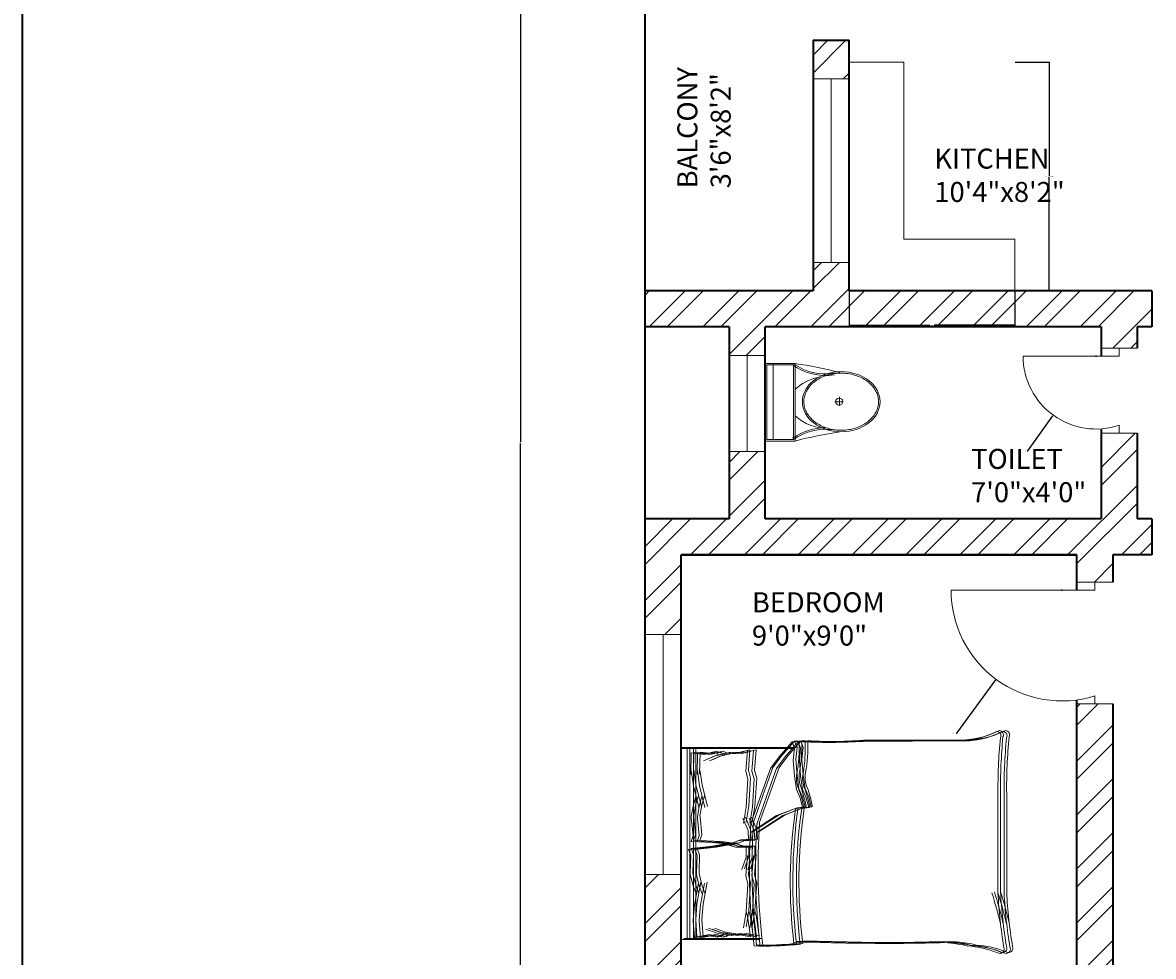
# Model space of a CAD drawing. Units: inches. Extents: x 1955 to 3324, y 980 to 3129.
# Tile 3 of 11: x 1955 to 2237, y 2048 to 2282. Entities that reach past the tile are written whole.
import ezdxf

# ---------------------------------------------------------------- set-up
doc = ezdxf.new("R2010")
doc.units = ezdxf.units.IN
for name, color, linetype, lineweight in [('A-ANNO-DIMS', 2, 'Continuous', 18), ('A-ANNO-TTLB', 7, 'Continuous', 35), ('A-AREA-IDEN', 7, 'Continuous', 18), ('A-DOOR', 3, 'Continuous', 18), ('A-FLOR-CASE', 8, 'Continuous', 18), ('A-FLOR-FIXT', 9, 'Continuous', 18), ('A-FURN', 8, 'Continuous', 18), ('A-GLAZ', 4, 'Continuous', 18), ('A-WALL', 7, 'Continuous', 35), ('A-WALL-PATT', 252, 'Continuous', 13)]:
    doc.layers.add(name, color=color, linetype=linetype, lineweight=lineweight)
doc.styles.get("Standard").update_dxf_attribs({"font": 'arial.ttf'})
doc.dimstyles.get("Standard").update_dxf_attribs({"dimtxt": 0.18, "dimasz": 0.18, "dimexe": 0.18, "dimexo": 0.0625, "dimgap": 0.09, "dimtad": 0, "dimtih": 1, "dimtoh": 1, "dimdec": 4, "dimzin": 0, "dimdsep": 46, "dimtxsty": 'Standard', "dimcen": 0.09, "dimadec": 0, "dimazin": 0, "dimtfac": 1, "dimtdec": 4, "dimtofl": 0, "dimtmove": 0, "dimatfit": 3, "dimfxl": 1, "dimtolj": 1, "dimtzin": 0, "dimarcsym": 0})

# ---------------------------------------------------------------- blocks, each defined once
blk = doc.blocks.new('A$C31115884')
for p, q in [((283.1, 497.7), (223.4, 497.7)), ((257.5, 466.4), (257.5, 523.2)), ((0, 200), (0, 0)), ((520, 200), (0, 200)), ((10, 190), (10, 10)), ((510, 190), (10, 190)), ((510, 10), (510, 190)), ((520, 0), (520, 200)), ((510, 54.5), (0, 54.5)), ((10, 10), (510, 10)), ((0, 0), (520, 0))]:
    blk.add_line(p, q)
blk.add_circle((255.6, 496.4), 23.6)
for centre, radius, start, end in [((2777.7, -204.6), 2807, 165.4549, 171.71327), ((-294.5, 403.3), 364.7, 324.20913, 9.34987), ((-294.5, 403.3), 374.7, 324.20913, 9.34987), ((805.8, 403.3), 364.7, 170.65013, 215.79087), ((3237, 905), 2807, 188.28673, 194.5451), ((139.5, 406.2), 293.5, 315.84364, 2.65635), ((805.8, 403.3), 374.7, 179.20365, 215.79087), ((383.6, 406.2), 293.5, 190.27735, 224.15636)]:
    blk.add_arc(centre, radius, start, end)
blk.add_ellipse((256.2, 509.9), major_axis=(0, -260.7), ratio=0.772727)
blk.add_open_spline([(256.2, 259.2), (263.1, 259.2), (270, 259.7), (287.8, 262.3), (298.7, 265.1), (319.9, 273.1), (330.2, 278.4), (350.1, 291.1), (359.7, 298.7), (377.7, 315.9), (386.2, 325.5), (401.7, 346.6), (408.8, 358.1), (421.3, 382.5), (426.8, 395.5), (435.9, 422.4), (439.5, 436.4), (444.8, 465.1), (446.5, 479.7), (447.9, 509.2), (447.6, 524), (445, 553.3), (442.7, 567.8), (436.3, 596), (432.1, 609.7), (421.9, 636), (416, 648.6), (402.5, 672.1), (395, 683), (378.6, 703), (369.8, 712.1), (351.1, 728), (341.3, 734.8), (320.9, 746.2), (310.4, 750.7), (288.9, 757.3), (278, 759.4), (256, 761), (245, 760.6), (223.1, 757.2), (212.3, 754.3), (191.1, 746.1), (180.8, 740.7), (160.9, 727.8), (151.4, 720.1), (133.5, 702.7), (125.1, 693), (109.6, 671.7), (102.6, 660.2), (90.2, 635.7), (84.9, 622.7), (76, 595.6), (72.4, 581.6), (67.2, 552.9), (65.6, 538.2), (64.4, 508.8), (64.8, 494), (67.5, 464.7), (69.9, 450.2), (76.6, 422), (80.8, 408.3), (91.1, 382.2), (97.2, 369.7), (110.8, 346.3), (118.4, 335.4), (134.8, 315.6), (143.7, 306.7), (162.4, 290.9), (172.3, 284.2), (192.8, 273), (203.3, 268.6), (224.8, 262.2), (235.8, 260.2), (249.9, 259.3), (253, 259.2), (256.2, 259.2)], degree=3, knots=[0, 0, 0, 0, 0.110105, 0.110105, 0.285049, 0.285049, 0.459994, 0.459994, 0.634938, 0.634938, 0.809882, 0.809882, 0.984827, 0.984827, 1.159771, 1.159771, 1.334715, 1.334715, 1.50966, 1.50966, 1.684604, 1.684604, 1.859549, 1.859549, 2.034493, 2.034493, 2.209437, 2.209437, 2.384382, 2.384382, 2.559326, 2.559326, 2.73427, 2.73427, 2.909215, 2.909215, 3.084159, 3.084159, 3.259103, 3.259103, 3.434048, 3.434048, 3.608992, 3.608992, 3.783936, 3.783936, 3.958881, 3.958881, 4.133825, 4.133825, 4.30877, 4.30877, 4.483714, 4.483714, 4.658658, 4.658658, 4.833603, 4.833603, 5.008547, 5.008547, 5.183491, 5.183491, 5.358436, 5.358436, 5.53338, 5.53338, 5.708324, 5.708324, 5.883269, 5.883269, 6.058213, 6.058213, 6.233158, 6.233158, 6.283185, 6.283185, 6.283185, 6.283185])
blk = doc.blocks.new('BED-WITH-PILLOWS')
for p, q in [((3.48, 63.33), (3.48, 81.44)), ((3.48, 63.33), (3.48, 81.44)), ((51.27, 81.44), (3.48, 81.44)), ((3.48, 79.91), (51.27, 79.91)), ((3.48, 79.91), (51.27, 79.91)), ((3.7, 62.69), (3.7, 80.8)), ((3.7, 62.69), (3.7, 80.8)), ((3.7, 79.27), (51.49, 79.27)), ((3.7, 79.27), (51.49, 79.27)), ((24.54, 78.99), (25.98, 79.57)), ((24.54, 78.99), (25.98, 79.57)), ((25.98, 79.57), (26.56, 74.22)), ((25.98, 79.57), (26.56, 74.22)), ((51.27, 81.44), (51.27, 54.83)), ((51.27, 81.44), (51.27, 54.83)), ((51.27, 81.44), (51.49, 81.44)), ((51.49, 81.44), (51.49, 80.8)), ((51.49, 80.8), (51.49, 54.19)), ((51.49, 80.8), (51.49, 54.19)), ((3.89, 78.13), (4.47, 74.95)), ((3.9, 78.11), (8.18, 78.43)), ((3.9, 78.11), (8.18, 78.43)), ((3.9, 78.13), (4.47, 74.95)), ((4.12, 77.49), (4.7, 74.31)), ((4.12, 77.49), (4.7, 74.31)), ((4.13, 77.47), (8.41, 77.8)), ((4.13, 77.47), (8.41, 77.8)), ((8.18, 78.43), (8.29, 78.42)), ((8.18, 78.43), (8.29, 78.42)), ((8.29, 78.42), (12.11, 78.13)), ((8.29, 78.42), (12.11, 78.13)), ((8.41, 77.8), (8.51, 77.78)), ((8.41, 77.8), (8.51, 77.78)), ((8.51, 77.78), (12.34, 77.49)), ((8.51, 77.78), (12.34, 77.49)), ((12.11, 78.13), (17.6, 77.12)), ((12.11, 78.13), (17.6, 77.12)), ((12.34, 77.49), (17.83, 76.48)), ((12.34, 77.49), (17.83, 76.48)), ((14.86, 77.69), (16.88, 78.42)), ((14.86, 77.69), (16.88, 78.42)), ((15.08, 77.05), (17.11, 77.78)), ((15.08, 77.05), (17.11, 77.78)), ((16.88, 78.42), (19.77, 79.14)), ((16.88, 78.42), (19.77, 79.14)), ((17.11, 77.78), (20, 78.5)), ((17.11, 77.78), (20, 78.5)), ((19.77, 79.14), (20.09, 79.14)), ((19.77, 79.14), (20.09, 79.14)), ((20, 78.5), (20.32, 78.5)), ((20, 78.5), (20.32, 78.5)), ((20.09, 79.14), (24.54, 78.99)), ((20.09, 79.14), (24.54, 78.99)), ((20.32, 78.5), (24.77, 78.36)), ((20.32, 78.5), (24.77, 78.36)), ((24.77, 78.36), (26.21, 78.93)), ((24.77, 78.36), (26.21, 78.93)), ((26.21, 78.93), (26.79, 73.58)), ((26.21, 78.93), (26.79, 73.58)), ((27.98, 78.95), (27.73, 73.58)), ((27.98, 78.95), (27.73, 73.58)), ((28.21, 78.31), (27.96, 72.94)), ((28.21, 78.31), (27.96, 72.94)), ((29.46, 78.46), (27.98, 78.95)), ((29.46, 78.46), (27.98, 78.95)), ((29.68, 77.83), (28.21, 78.31)), ((29.68, 77.83), (28.21, 78.31)), ((33.88, 78.89), (29.46, 78.46)), ((33.88, 78.89), (29.46, 78.46)), ((34.11, 78.25), (29.68, 77.83)), ((34.11, 78.25), (29.68, 77.83)), ((34.21, 78.91), (33.88, 78.89)), ((34.2, 78.91), (33.88, 78.89)), ((34.43, 78.27), (34.11, 78.25)), ((34.43, 78.27), (34.11, 78.25)), ((37.14, 78.36), (34.2, 78.91)), ((37.14, 78.36), (34.21, 78.91)), ((37.36, 77.73), (34.43, 78.27)), ((37.36, 77.73), (34.43, 78.27)), ((41.91, 78.37), (36.5, 77.02)), ((41.91, 78.37), (36.5, 77.02)), ((42.14, 77.73), (36.72, 76.38)), ((42.14, 77.73), (36.72, 76.38)), ((39.2, 77.77), (37.14, 78.36)), ((39.2, 77.77), (37.14, 78.36)), ((39.43, 77.13), (37.36, 77.73)), ((39.43, 77.13), (37.36, 77.73)), ((45.71, 78.9), (41.91, 78.37)), ((45.71, 78.9), (41.91, 78.37)), ((45.94, 78.26), (42.14, 77.73)), ((45.94, 78.26), (42.14, 77.73)), ((50.11, 78.89), (44.71, 78.98)), ((44.71, 78.98), (45.71, 78.9)), ((50.11, 78.89), (44.71, 78.98)), ((44.71, 78.98), (45.71, 78.9)), ((50.34, 78.25), (44.94, 78.34)), ((44.94, 78.34), (45.94, 78.26)), ((50.34, 78.25), (44.94, 78.34)), ((44.94, 78.34), (45.94, 78.26)), ((50.11, 78.89), (49.73, 75.68)), ((50.11, 78.89), (49.73, 75.68)), ((50.34, 78.25), (49.96, 75.04)), ((50.34, 78.25), (49.96, 75.04)), ((4.47, 74.95), (4.04, 72.34)), ((4.47, 74.95), (4.04, 72.34)), ((4.7, 74.31), (4.27, 71.7)), ((4.7, 74.31), (4.27, 71.7)), ((5.05, 72.49), (6.06, 75.24)), ((5.05, 72.49), (6.06, 75.24)), ((5.28, 71.85), (6.29, 74.6)), ((5.28, 71.85), (6.29, 74.6)), ((26.56, 74.22), (27.14, 71.04)), ((26.56, 74.22), (27.14, 71.04)), ((26.79, 73.58), (27.37, 70.4)), ((26.79, 73.58), (27.37, 70.4)), ((27.73, 73.58), (27.36, 70.37)), ((27.73, 73.58), (27.36, 70.37)), ((49.31, 73.19), (48.13, 75.86)), ((49.31, 73.19), (48.13, 75.86)), ((49.54, 72.55), (48.36, 75.23)), ((49.54, 72.55), (48.36, 75.23)), ((49.73, 75.68), (50.33, 73.11)), ((49.73, 75.68), (50.33, 73.11)), ((49.96, 75.04), (50.56, 72.47)), ((49.96, 75.04), (50.56, 72.47)), ((4.04, 72.34), (4.62, 71.33)), ((4.04, 72.34), (4.62, 71.33)), ((4.27, 71.7), (4.85, 70.69)), ((4.27, 71.7), (4.85, 70.69)), ((4.47, 68.87), (5.05, 72.49)), ((4.47, 68.87), (5.05, 72.49)), ((4.7, 68.23), (5.28, 71.85)), ((4.7, 68.23), (5.28, 71.85)), ((27.14, 71.04), (27.14, 69.74)), ((27.14, 71.04), (27.14, 69.74)), ((27.96, 72.94), (27.58, 69.73)), ((27.96, 72.94), (27.58, 69.73)), ((50.11, 69.61), (49.31, 73.19)), ((50.11, 69.61), (49.31, 73.19)), ((50.34, 68.98), (49.54, 72.55)), ((50.34, 68.98), (49.54, 72.55)), ((50.33, 73.11), (49.81, 72.06)), ((50.33, 73.11), (49.82, 72.06)), ((50.56, 72.47), (50.04, 71.42)), ((50.56, 72.47), (50.04, 71.42)), ((4.76, 67.28), (4.47, 68.87)), ((4.76, 67.28), (4.47, 68.87)), ((4.99, 66.64), (4.7, 68.23)), ((4.99, 66.64), (4.7, 68.23)), ((27.14, 69.74), (26.56, 67.86)), ((27.14, 69.74), (26.56, 67.86)), ((27.37, 69.1), (26.79, 67.22)), ((27.37, 69.1), (26.79, 67.22)), ((27.36, 70.37), (27.44, 69.07)), ((27.36, 70.37), (27.44, 69.07)), ((27.37, 70.4), (27.37, 69.1)), ((27.37, 70.4), (27.37, 69.1)), ((27.44, 69.07), (28.13, 67.23)), ((27.44, 69.07), (28.13, 67.23)), ((27.58, 69.73), (27.66, 68.43)), ((27.58, 69.73), (27.66, 68.43)), ((27.66, 68.43), (28.36, 66.59)), ((27.66, 68.43), (28.36, 66.59)), ((49.92, 68.01), (50.11, 69.61)), ((49.92, 68.01), (50.11, 69.61)), ((50.7, 64.87), (49.92, 68.01)), ((50.7, 64.87), (49.92, 68.01)), ((50.15, 67.37), (50.34, 68.98)), ((50.15, 67.37), (50.34, 68.98)), ((4.18, 64.1), (4.76, 67.28)), ((4.18, 64.1), (4.76, 67.28)), ((4.41, 63.46), (4.99, 66.64)), ((4.41, 63.46), (4.99, 66.64)), ((6.38, 65.81), (10.41, 65.15)), ((6.38, 65.81), (10.41, 65.15)), ((6.61, 65.18), (10.64, 64.51)), ((6.61, 65.18), (10.64, 64.51)), ((10.41, 65.15), (9.28, 64.83)), ((10.41, 65.15), (9.28, 64.83)), ((10.41, 65.15), (17.42, 64.72)), ((10.41, 65.15), (17.42, 64.72)), ((17.42, 64.72), (19.38, 65.27)), ((17.42, 64.72), (19.38, 65.27)), ((19.38, 65.27), (24.52, 64.87)), ((19.38, 65.27), (24.52, 64.87)), ((24.1, 65.18), (20.96, 66.27)), ((24.1, 65.18), (20.96, 66.27)), ((24.33, 64.54), (21.19, 65.63)), ((24.33, 64.54), (21.19, 65.63)), ((26.56, 65.18), (24.1, 65.18)), ((26.56, 65.18), (24.1, 65.18)), ((26.56, 67.86), (26.56, 65.18)), ((26.56, 67.86), (26.56, 65.18)), ((26.79, 67.22), (26.79, 64.54)), ((26.79, 67.22), (26.79, 64.54)), ((28.13, 67.23), (28.3, 64.55)), ((28.13, 67.23), (28.3, 64.55)), ((28.36, 66.59), (28.53, 63.91)), ((28.36, 66.59), (28.53, 63.91)), ((30.75, 64.7), (33.82, 65.99)), ((30.75, 64.7), (33.82, 65.99)), ((30.98, 64.06), (34.05, 65.35)), ((30.98, 64.06), (34.05, 65.35)), ((32.56, 65.81), (36.6, 65.15)), ((32.56, 65.81), (36.6, 65.15)), ((32.79, 65.18), (36.83, 64.51)), ((32.79, 65.18), (36.82, 64.51)), ((36.6, 65.15), (43.61, 64.72)), ((36.6, 65.15), (43.61, 64.72)), ((43.61, 64.72), (45.57, 65.27)), ((43.61, 64.72), (45.57, 65.27)), ((45.57, 65.27), (50.7, 64.87)), ((45.57, 65.27), (50.7, 64.87)), ((50.93, 64.23), (50.15, 67.37)), ((50.93, 64.23), (50.15, 67.37)), ((9.28, 64.83), (4.18, 64.1)), ((9.28, 64.83), (4.18, 64.1)), ((9.51, 64.19), (4.41, 63.46)), ((9.51, 64.19), (4.41, 63.46)), ((10.64, 64.51), (9.51, 64.19)), ((10.64, 64.51), (9.51, 64.19)), ((10.64, 64.51), (17.65, 64.08)), ((10.64, 64.51), (17.65, 64.08)), ((17.65, 64.08), (19.61, 64.63)), ((17.65, 64.08), (19.61, 64.63)), ((19.61, 64.63), (24.74, 64.23)), ((19.61, 64.63), (24.74, 64.23)), ((26.79, 64.54), (24.33, 64.54)), ((26.79, 64.54), (24.33, 64.54)), ((28.3, 64.55), (30.75, 64.7)), ((28.3, 64.55), (30.75, 64.7)), ((28.53, 63.91), (30.98, 64.06)), ((28.53, 63.91), (30.98, 64.06)), ((30.26, 64.06), (34.45, 57.57)), ((30.26, 64.06), (34.45, 57.57)), ((30.49, 63.42), (34.68, 56.93)), ((30.49, 63.42), (34.68, 56.93)), ((40.64, 61.13), (32.31, 64.06)), ((40.64, 61.13), (32.31, 64.06)), ((40.87, 60.49), (32.53, 63.42)), ((40.87, 60.49), (32.54, 63.42)), ((36.82, 64.51), (43.83, 64.08)), ((36.83, 64.51), (43.84, 64.08)), ((43.83, 64.08), (45.8, 64.63)), ((43.84, 64.08), (45.8, 64.63)), ((45.8, 64.63), (50.93, 64.23)), ((45.8, 64.63), (50.93, 64.23)), ((46.22, 59.11), (40.64, 61.13)), ((46.22, 59.11), (40.64, 61.13)), ((46.45, 58.48), (40.87, 60.49)), ((46.45, 58.48), (40.87, 60.49)), ((34.45, 57.57), (36.15, 53.08)), ((34.45, 57.57), (36.15, 53.08)), ((34.68, 56.93), (36.38, 52.44)), ((34.68, 56.93), (36.38, 52.44)), ((49.16, 56.95), (46.22, 59.11)), ((49.16, 56.95), (46.22, 59.11)), ((49.39, 56.31), (46.45, 58.48)), ((49.39, 56.31), (46.45, 58.48)), ((52.87, 53.7), (49.16, 56.95)), ((52.87, 53.7), (49.16, 56.95)), ((53.1, 53.06), (49.39, 56.31)), ((53.1, 53.06), (49.39, 56.31)), ((36.15, 53.08), (36.46, 51.07)), ((36.15, 53.08), (36.46, 51.07)), ((36.38, 52.44), (36.69, 50.43)), ((36.38, 52.44), (36.69, 50.43)), ((36.46, 51.07), (38.94, 51.69)), ((36.46, 51.07), (38.94, 51.69)), ((36.69, 50.43), (39.17, 51.05)), ((36.69, 50.43), (39.17, 51.05)), ((38.94, 51.69), (40.95, 52.61)), ((38.94, 51.69), (40.95, 52.61)), ((39.17, 51.05), (41.18, 51.97)), ((39.17, 51.05), (41.18, 51.97)), ((40.95, 52.61), (44.36, 53.08)), ((40.95, 52.61), (44.36, 53.08)), ((41.18, 51.97), (44.59, 52.44)), ((41.18, 51.97), (44.59, 52.44)), ((44.36, 53.08), (48.23, 53.39)), ((44.36, 53.08), (48.23, 53.39)), ((44.59, 52.44), (48.46, 52.75)), ((44.59, 52.44), (48.46, 52.75)), ((48.23, 53.39), (51.33, 53.08)), ((48.23, 53.39), (51.33, 53.08)), ((48.46, 52.75), (51.56, 52.44)), ((48.46, 52.75), (51.56, 52.44)), ((51.33, 53.08), (52.87, 53.7)), ((51.33, 53.08), (52.87, 53.7)), ((51.56, 52.44), (53.1, 53.06)), ((51.56, 52.44), (53.1, 53.06)), ((52.95, 51.95), (52.87, 53.7, 3.87)), ((52.95, 51.95), (52.87, 53.7, 3.87)), ((53.18, 51.31), (53.1, 53.06, 3.87)), ((53.18, 51.31), (53.1, 53.06, 3.87)), ((15.06, 2.2), (39.68, 2.2)), ((15.06, 2.2), (39.68, 2.2)), ((15.29, 1.56), (39.91, 1.56)), ((15.29, 1.56), (39.91, 1.56))]:
    blk.add_line(p, q)
for centre, radius, start, end in [((85.16, 61.35), 83.31, 178.7218, 185.604), ((85.16, 61.35), 83.31, 178.7218, 185.604), ((21.36, -100.61), 164.97, 86.0865, 96.7821), ((21.36, -100.61), 164.97, 86.0865, 96.7821), ((85.39, 60.71), 83.31, 178.7218, 185.604), ((85.39, 60.71), 83.31, 178.7218, 185.604), ((21.59, -101.25), 164.97, 86.0865, 96.7821), ((21.59, -101.25), 164.97, 86.0865, 96.7821), ((17.76, -74.87), 129.02, 81.7845, 96.9006), ((17.76, -74.87), 129.02, 81.7845, 96.9006), ((17.98, -75.51), 129.02, 81.7845, 96.9006), ((17.98, -75.51), 129.02, 81.7845, 96.9006), ((-167.31, 50.27), 170.11, 358.4762, 1.0082), ((-167.31, 50.27), 170.11, 358.4762, 1.0082), ((-167.08, 49.63), 170.11, 358.4762, 1.0082), ((-167.08, 49.63), 170.11, 358.4762, 1.0082), ((36.64, 51), 0.185, 160.2464, 271.1377), ((36.64, 51), 0.185, 160.2464, 271.1377), ((31.15, 79.96), 29.65, 280.6617, 289.8806), ((31.15, 79.96), 29.65, 280.6617, 289.8806), ((31.38, 79.32), 29.65, 280.6617, 289.8806), ((31.38, 79.32), 29.65, 280.6617, 289.8806), ((43.74, 46.38), 6.22, 78.6608, 113.7384), ((43.74, 46.38), 6.22, 78.6608, 113.7384), ((43.97, 45.74), 6.22, 78.6608, 113.7384), ((43.97, 45.74), 6.22, 78.6608, 113.7384), ((51.33, 88.1), 36.18, 259.8763, 272.5657), ((51.33, 88.1), 36.18, 259.8763, 272.5657), ((51.56, 87.46), 36.18, 259.8763, 272.5657), ((51.56, 87.46), 36.18, 259.8763, 272.5657), ((182.27, 45.13), 129.5, 176.9791, 183.8365), ((182.27, 45.13), 129.5, 176.9791, 183.8365), ((182.49, 44.49), 129.5, 176.9791, 183.8365), ((182.49, 44.49), 129.5, 176.9791, 183.8365), ((36.87, 50.36), 0.185, 160.2464, 271.1377), ((36.86, 50.36), 0.185, 160.2464, 271.1377), ((484.82, 30.83), 482.31, 178.2277, 181.7185), ((484.82, 30.83), 482.31, 178.2277, 181.7185), ((485.05, 30.19), 482.31, 178.2277, 181.7185), ((485.05, 30.19), 482.31, 178.2277, 181.7185), ((-4508.74, 13.62), 4561.86, 0.00217, 0.28689), ((-4508.74, 13.62), 4561.86, 0.00217, 0.28689), ((-4508.51, 12.98), 4561.86, 0.00217, 0.28689), ((-4508.51, 12.98), 4561.86, 0.00217, 0.28689), ((-26.9, 16.93), 29.63, 346.0648, 358.9113), ((-26.9, 16.93), 29.63, 346.0648, 358.9113), ((-26.67, 16.29), 29.63, 346.0648, 358.9113), ((-26.67, 16.29), 29.63, 346.0648, 358.9113), ((76.16, 12.78), 23.07, 177.4714, 206.4681), ((76.16, 12.78), 23.07, 177.4714, 206.4681), ((76.39, 12.14), 23.07, 177.4714, 206.4681), ((76.39, 12.14), 23.07, 177.4714, 206.4681), ((-21.66, 11.17), 23.56, 337.9751, 356.652), ((-21.66, 11.17), 23.56, 337.9751, 356.652), ((-21.43, 10.53), 23.56, 337.9751, 356.652), ((-21.43, 10.53), 23.56, 337.9751, 356.652), ((-17.22, 105.16), 106.46, 283.3832, 287.7053), ((-17.22, 105.16), 106.46, 283.3832, 287.7053), ((-16.99, 104.52), 106.46, 283.3832, 287.7053), ((-16.99, 104.52), 106.46, 283.3832, 287.7053), ((1.09, 1.73), 1.09, 146.1736, 293.4781), ((1.09, 1.73), 1.09, 146.1736, 293.4781), ((1.32, 1.09), 1.09, 146.1736, 293.4781), ((1.32, 1.09), 1.09, 146.1736, 293.4781), ((21.43, -119.39), 121.76, 92.9958, 99.4091), ((21.43, -119.39), 121.76, 92.9958, 99.4091), ((21.66, -120.03), 121.76, 92.9958, 99.4091), ((21.66, -120.03), 121.76, 92.9958, 99.4091), ((41.15, -130.83), 133.04, 84.4998, 90.6351), ((41.15, -130.83), 133.04, 84.4998, 90.6351), ((41.38, -131.47), 133.04, 84.4998, 90.6351), ((41.38, -131.47), 133.04, 84.4998, 90.6351), ((54.41, 2.57), 1.1, 242.6588, 356.02), ((54.41, 2.57), 1.1, 242.6588, 356.02), ((54.64, 1.93), 1.1, 242.6588, 356.02), ((54.64, 1.93), 1.1, 242.6588, 356.02)]:
    blk.add_arc(centre, radius, start, end)
blk = doc.blocks.new('DOOR-WC-W')
for p, q in [((28.5, 21.31), (19.5, 21.31)), ((19.5, 21.31), (24, 21.31)), ((24, 21.31), (24, 19.31)), ((24, 19.31), (0, 19.31)), ((19.5, 0), (28.5, 0)), ((24, 0), (24, 2)), ((28.5, 0), (24, 0))]:
    blk.add_line(p, q)
blk.add_arc((18.25, 19.31), 18.25, 180, 288.3841)
blk = doc.blocks.new('DOOR-BED-W')
for p, q in [((36, 28.47), (0, 28.47)), ((40.5, 30.47), (31.5, 30.47)), ((31.5, 30.47), (36, 30.47)), ((36, 30.47), (36, 28.47)), ((31.5, 0), (40.5, 0)), ((36, 0), (36, 2)), ((40.5, 0), (36, 0))]:
    blk.add_line(p, q)
blk.add_arc((27.73, 28.47), 27.73, 180, 287.3494)
blk = doc.blocks.new('WIN-PLAN-60-A')
for p, q in [((0, 60), (9, 60)), ((9, 60), (4.5, 60)), ((4.5, 60), (4.5, 0)), ((4.5, 0), (0, 0)), ((0, 0), (9, 0))]:
    blk.add_line(p, q)
blk = doc.blocks.new('WIN-PLAN-24-A')
for p, q in [((0, 9), (0, 0)), ((24, 4.5), (24, 9)), ((24, 9), (24, 0)), ((0, 0), (0, 4.5)), ((0, 4.5), (24, 4.5))]:
    blk.add_line(p, q)
blk = doc.blocks.new('WIN-PLAN-46')
for p, q in [((0, 45.87), (9, 45.87)), ((9, 45.87), (4.5, 45.87)), ((4.5, 45.87), (4.5, 0)), ((4.5, 0), (0, 0)), ((0, 0), (9, 0))]:
    blk.add_line(p, q)
blk = doc.blocks.new('COUNTER-L-W')
for p, q in [((0, 57.19), (13.72, 57.19)), ((13.72, 57.19), (13.72, 12.97)), ((13.72, 12.97), (41.47, 12.97)), ((41.47, 12.97), (41.47, 0))]:
    blk.add_line(p, q)
blk = doc.blocks.new('*D81')
at = {"layer": 'A-ANNO-DIMS', "color": 0, "lineweight": -2, "transparency": 16777216}
for p, q in [((2202.74, 2271.7), (2211.44, 2271.7)), ((2211.26, 2271.52), (2211.26, 2243.28)), ((2211.26, 2214.68), (2211.26, 2242.92)), ((2202.74, 2214.5), (2211.44, 2214.5))]:
    blk.add_line(p, q, dxfattribs=at)
at = {"layer": 'A-ANNO-DIMS', "color": 0, "transparency": 16777216}
for points in [[(2211.23, 2271.52), (2211.29, 2271.52), (2211.26, 2271.7)], [(2211.23, 2214.68), (2211.29, 2214.68), (2211.26, 2214.5)]]:
    blk.add_solid(points, dxfattribs=at)
at = {"layer": 'Defpoints', "color": 0, "transparency": 16777216}
for p in [(2202.68, 2271.7), (2211.26, 2271.7), (2202.68, 2214.5)]:
    blk.add_point(p, dxfattribs=at)
at = {"layer": 'A-ANNO-DIMS', "color": 0, "transparency": 16777216, "insert": (2211.26, 2243.1), "char_height": 0.18, "attachment_point": 5}
blk.add_mtext('\\A1;COUNTER 57 TYP.', dxfattribs=at)
blk = doc.blocks.new('*D82')
at = {"layer": 'A-ANNO-DIMS', "color": 0, "lineweight": -2, "transparency": 16777216}
for p, q in [((2161.21, 2214.44), (2161.21, 2205.74)), ((2202.68, 2214.44), (2202.68, 2205.74)), ((2161.39, 2205.92), (2181.41, 2205.92)), ((2202.5, 2205.92), (2182.48, 2205.92))]:
    blk.add_line(p, q, dxfattribs=at)
at = {"layer": 'A-ANNO-DIMS', "color": 0, "transparency": 16777216}
for points in [[(2161.39, 2205.95), (2161.39, 2205.89), (2161.21, 2205.92)], [(2202.5, 2205.95), (2202.5, 2205.89), (2202.68, 2205.92)]]:
    blk.add_solid(points, dxfattribs=at)
at = {"layer": 'Defpoints', "color": 0, "transparency": 16777216}
for p in [(2161.21, 2214.5), (2202.68, 2214.5), (2202.68, 2205.92)]:
    blk.add_point(p, dxfattribs=at)
at = {"layer": 'A-ANNO-DIMS', "color": 0, "transparency": 16777216, "insert": (2181.94, 2205.92), "char_height": 0.18, "attachment_point": 5}
blk.add_mtext('\\A1;41 TYP.', dxfattribs=at)
blk = doc.blocks.new('*D92')
at = {"layer": 'A-ANNO-DIMS', "color": 0, "lineweight": -2, "transparency": 16777216}
for p, q in [((2110.15, 2456.5), (2078.88, 2456.5)), ((2079.06, 2456.32), (2079.06, 2176.69)), ((2079.06, 1896.68), (2079.06, 2176.32)), ((2110.15, 1896.5), (2078.88, 1896.5))]:
    blk.add_line(p, q, dxfattribs=at)
at = {"layer": 'A-ANNO-DIMS', "color": 0, "transparency": 16777216}
for points in [[(2079.03, 2456.32), (2079.09, 2456.32), (2079.06, 2456.5)], [(2079.03, 1896.68), (2079.09, 1896.68), (2079.06, 1896.5)]]:
    blk.add_solid(points, dxfattribs=at)
at = {"layer": 'Defpoints', "color": 0, "transparency": 16777216}
for p in [(2079.06, 2456.5), (2110.21, 2456.5), (2110.21, 1896.5)]:
    blk.add_point(p, dxfattribs=at)
at = {"layer": 'A-ANNO-DIMS', "color": 0, "transparency": 16777216, "insert": (2079.06, 2176.5), "char_height": 0.18, "attachment_point": 5}
blk.add_mtext('\\A1;560', dxfattribs=at)
blk = doc.blocks.new('*D142')
at = {"layer": 'A-ANNO-DIMS', "color": 0, "lineweight": -2, "transparency": 16777216}
for p, q in [((2214.35, 2139.73), (2214.53, 2139.73)), ((2214.44, 2139.64), (2214.44, 2139.82)), ((2188.16, 2103.98), (2197.91, 2117.24)), ((2187.98, 2103.98), (2188.16, 2103.98))]:
    blk.add_line(p, q, dxfattribs=at)
at = {"layer": 'A-ANNO-DIMS', "color": 0, "transparency": 16777216}
blk.add_solid([(2197.88, 2117.26), (2197.93, 2117.22), (2198.01, 2117.38)], dxfattribs=at)
at = {"layer": 'Defpoints', "color": 0, "transparency": 16777216}
for p in [(2214.44, 2139.73), (2198.01, 2117.38)]:
    blk.add_point(p, dxfattribs=at)
at = {"layer": 'A-ANNO-DIMS', "color": 0, "transparency": 16777216, "insert": (2187.5, 2103.98), "char_height": 0.18, "attachment_point": 5}
blk.add_mtext('\\A1;R27.73', dxfattribs=at)
blk = doc.blocks.new('*D147')
at = {"layer": 'A-ANNO-DIMS', "color": 0, "lineweight": -2, "transparency": 16777216}
for p, q in [((2222.89, 2198.23), (2223.07, 2198.23)), ((2222.98, 2198.14), (2222.98, 2198.32)), ((2205.9, 2174.56), (2212.2, 2183.29)), ((2205.72, 2174.56), (2205.9, 2174.56))]:
    blk.add_line(p, q, dxfattribs=at)
at = {"layer": 'A-ANNO-DIMS', "color": 0, "transparency": 16777216}
blk.add_solid([(2212.18, 2183.31), (2212.23, 2183.27), (2212.31, 2183.43)], dxfattribs=at)
at = {"layer": 'Defpoints', "color": 0, "transparency": 16777216}
for p in [(2222.98, 2198.23), (2212.31, 2183.43)]:
    blk.add_point(p, dxfattribs=at)
at = {"layer": 'A-ANNO-DIMS', "color": 0, "transparency": 16777216, "insert": (2205.18, 2174.56), "char_height": 0.18, "attachment_point": 5}
blk.add_mtext('\\A1;R18.246', dxfattribs=at)

msp = doc.modelspace()

# ---------------------------------------------------------------- hatches: boundary and pattern name
at = {"layer": 'A-WALL-PATT'}
h = msp.add_hatch(dxfattribs=at)
h.set_pattern_fill('ANSI32', color=256)
h.paths.add_polyline_path([(2361.4775, 2456.5037), (2270.2755, 2456.5037), (2270.2755, 2447.5037), (2285.7102, 2447.5037), (2285.7102, 2363.5037), (2281.1795, 2363.5037), (2281.1795, 2359.0037), (2290.2102, 2359.0037), (2290.2102, 2447.5037), (2361.4775, 2447.5037), (2361.4775, 2452.0037)])
h.paths.add_polyline_path([(2246.2755, 2456.5037), (2197.6809, 2456.5037), (2197.6809, 2447.5037), (2233.2102, 2447.5037), (2233.2102, 2355.6044), (2237.7102, 2355.6044), (2237.7102, 2447.5037), (2246.2755, 2447.5037)], flags=17)
h.paths.add_polyline_path([(2137.6809, 2456.5037), (2110.2102, 2456.5037), (2110.2102, 2312.5037), (2152.2102, 2312.5037), (2281.2102, 2312.5037), (2281.2102, 2107.6185), (2290.2102, 2107.6185), (2290.2102, 2267.9289), (2329.216, 2267.9289), (2329.216, 2272.4289), (2329.216, 2276.9289), (2290.2102, 2276.9289), (2290.2102, 2321.5037), (2281.2102, 2321.5037), (2119.2102, 2321.5037), (2119.2102, 2447.5037), (2137.6809, 2447.5037)])
h.paths.add_polyline_path([(2515.2102, 2456.5037), (2421.4775, 2456.5037), (2421.4775, 2447.5037), (2506.2102, 2447.5037), (2506.2102, 2415.6626), (2515.2102, 2415.6626)])
h.paths.add_polyline_path([(2515.2102, 2355.6626), (2506.2102, 2355.6626), (2506.2102, 2321.5037), (2424.9282, 2321.5037), (2424.9282, 2312.5037), (2461.2102, 2312.5037), (2470.2102, 2312.5037), (2515.2102, 2312.5037)])
h.paths.add_polyline_path([(2515.2102, 2232.5037), (2470.2102, 2232.5037), (2470.2102, 2237.3759), (2465.7102, 2237.3759), (2461.2102, 2237.3759), (2461.2102, 2232.5037), (2377.2219, 2232.5037), (2377.2219, 2321.5037), (2368.2219, 2321.5037), (2368.2219, 2276.9289), (2359.3802, 2276.9289), (2359.3802, 2272.4289), (2359.3802, 2267.9289), (2368.2219, 2267.9289), (2368.2219, 2223.5037), (2377.2219, 2223.5037), (2461.2102, 2223.5037), (2506.2102, 2223.5037), (2506.2102, 2129.5037), (2461.2102, 2129.5037), (2387.2102, 2129.5037), (2368.2219, 2129.5037), (2368.2219, 2056.4936), (2361.0095, 2056.4936), (2361.0095, 2051.9936), (2361.0095, 2047.4936), (2368.2219, 2047.4936), (2368.2219, 2031.5037), (2377.2219, 2031.5037), (2377.2219, 2120.5037), (2461.2102, 2120.5037), (2461.2102, 2112.7921), (2470.2102, 2112.7921), (2470.2102, 2120.5037), (2515.2102, 2120.5037), (2515.2102, 2129.5037)])
h.paths.add_polyline_path([(2470.2102, 2277.1758), (2461.2102, 2277.1758), (2461.2102, 2272.5037), (2461.2102, 2270.2549), (2470.2102, 2270.2549), (2470.2102, 2272.5037)], flags=17)
h.paths.add_polyline_path([(2515.2102, 2040.5037), (2470.2102, 2040.5037), (2417.8264, 2040.5037), (2417.8264, 2031.5037), (2506.2102, 2031.5037), (2506.2102, 2005.3639), (2515.2102, 2005.3639)])
h.paths.add_polyline_path([(2506.2102, 1905.5037), (2402.6963, 1905.5037), (2402.6963, 1896.5037), (2506.2102, 1896.5037)])
h.paths.add_polyline_path([(2515.2102, 1945.3639), (2506.2102, 1945.3639), (2506.2102, 1905.5037), (2506.2102, 1896.5037), (2515.2102, 1896.5037)])
h.paths.add_polyline_path([(2342.6963, 1901.0037), (2342.6963, 1905.5037), (2273.4892, 1905.5037), (2273.4892, 1896.5037), (2342.6963, 1896.5037)])
h.paths.add_polyline_path([(2290.2102, 1994.0037), (2283.612, 1994.0037), (2283.612, 1991.7537), (2283.612, 1989.5037), (2285.7102, 1989.5037), (2285.7102, 1905.5037), (2290.2102, 1905.5037)])
h.paths.add_polyline_path([(2249.4892, 1905.5037), (2237.7102, 1905.5037), (2206.3617, 1905.5037), (2206.3617, 1896.5037), (2249.4892, 1896.5037), (2249.4892, 1901.0037)])
h.paths.add_polyline_path([(2237.7102, 1989.5037), (2261.7102, 1989.5037), (2261.7102, 1994.0037), (2237.7102, 1994.0037), (2237.7102, 1999.266), (2235.4602, 1999.266), (2233.2102, 1999.266), (2233.2102, 1994.0037), (2233.2102, 1905.5037), (2237.7102, 1905.5037)])
h.paths.add_polyline_path([(2119.2102, 1947.5144), (2110.2102, 1947.5144), (2110.2102, 1896.5037), (2119.2102, 1896.5037), (2146.3617, 1896.5037), (2146.3617, 1901.0037), (2146.3617, 1905.5037), (2119.2102, 1905.5037)])
h.paths.add_polyline_path([(2119.2102, 2068.6379), (2110.2102, 2068.6379), (2110.2102, 2007.5144), (2119.2102, 2007.5144), (2119.2102, 2031.5037), (2233.2102, 2031.5037), (2233.2102, 2027.9287), (2235.4602, 2027.9287), (2237.7102, 2027.9287), (2237.7102, 2031.5037), (2281.2102, 2031.5037), (2290.2102, 2031.5037), (2290.2102, 2047.4936), (2326.409, 2047.4936), (2326.409, 2056.4936), (2290.2102, 2056.4936), (2290.2102, 2071.2722), (2285.7102, 2071.2722), (2281.2102, 2071.2722), (2281.2102, 2040.5037), (2227.2102, 2040.5037), (2227.2102, 2111.2571), (2222.7102, 2111.2571), (2218.2102, 2111.2571), (2218.2102, 2040.5037), (2119.2102, 2040.5037)])
h.paths.add_polyline_path([(2236.9166, 2214.5037), (2161.2102, 2214.5037), (2161.2102, 2221.6488), (2152.2102, 2221.6488), (2152.2102, 2214.5037), (2110.2102, 2214.5037), (2110.2102, 2205.5037), (2131.2394, 2205.5037), (2131.2394, 2198.3478), (2140.2394, 2198.3478), (2140.2394, 2205.5037), (2224.2394, 2205.5037), (2224.2394, 2200.2317), (2228.7394, 2200.2317), (2233.2394, 2200.2317), (2233.2394, 2205.5037), (2236.9166, 2205.5037)], flags=17)
h.paths.add_polyline_path([(2236.9166, 2157.5037), (2233.2394, 2157.5037), (2233.2394, 2178.9172), (2228.7394, 2178.9172), (2224.2394, 2178.9172), (2224.2394, 2157.5037), (2140.2394, 2157.5037), (2140.2394, 2174.3478), (2131.2394, 2174.3478), (2131.2394, 2157.5037), (2110.2102, 2157.5037), (2110.2102, 2128.6379), (2119.2102, 2128.6379), (2119.2102, 2148.5037), (2218.2102, 2148.5037), (2218.2102, 2141.7262), (2222.7102, 2141.7262), (2227.2102, 2141.7262), (2227.2102, 2148.5037), (2236.9166, 2148.5037)], flags=0)
h.paths.add_polyline_path([(3084.7449, 2537.3808), (3212.7954, 2537.3808), (3212.7954, 2555.9271), (3084.7449, 2555.9271)], flags=9)
h.paths.add_polyline_path([(3068.7485, 2853.43), (3169.977, 2853.43), (3169.977, 2871.9764), (3068.7485, 2871.9764)], flags=9)
h.paths.add_polyline_path([(3074.1798, 2918.0252), (3126.4732, 2918.0252), (3126.4732, 2936.5716), (3074.1798, 2936.5716)], flags=9)
h.paths.add_polyline_path([(3073.0928, 2947.3127), (3199.0499, 2947.3127), (3199.0499, 2965.8591), (3073.0928, 2965.8591)], flags=9)
h.paths.add_polyline_path([(2733.8393, 2484.8678), (2879.7915, 2484.8678), (2879.7915, 2521.9606), (2733.8393, 2521.9606)], flags=9)
h.paths.add_polyline_path([(2204.9881, 2482.4168), (2355.1272, 2482.4168), (2355.1272, 2519.5095), (2204.9881, 2519.5095)], flags=9)
h.paths.add_polyline_path([(3062.1429, 2387.2466), (3079.3735, 2387.2466), (3079.3735, 2411.9751), (3062.1429, 2411.9751)], flags=9)
h.paths.add_polyline_path([(2190.1574, 2158.8439), (2219.315, 2158.8439), (2219.315, 2177.5013), (2190.1574, 2177.5013)], flags=25)
h.paths.add_polyline_path([(2213.6766, 1840.7276), (2405.0382, 1840.7276), (2405.0382, 1865.4561), (2213.6766, 1865.4561)], flags=9)
h.paths.add_polyline_path([(2180.5398, 2233.911), (2213.9471, 2233.911), (2213.9471, 2252.5683), (2180.5398, 2252.5683)], flags=25)
h.paths.add_polyline_path([(2134.4484, 2238.3973), (2134.4484, 2274.2807), (2115.791, 2274.2807), (2115.791, 2238.3973)], flags=25)
h.paths.add_polyline_path([(2135.1593, 2122.9991), (2173.7507, 2122.9991), (2173.7507, 2141.6565), (2135.1593, 2141.6565)], flags=25)
h.paths.add_polyline_path([(2129.8822, 2002.1912), (2168.4736, 2002.1912), (2168.4736, 2020.8486), (2129.8822, 2020.8486)], flags=9)
h.paths.add_polyline_path([(2239.6647, 1953.4107), (2268.8973, 1953.4107), (2268.8973, 1972.068), (2239.6647, 1972.068)], flags=9)
h.paths.add_polyline_path([(2352.8562, 1951.2904), (2402.1775, 1951.2904), (2402.1775, 1969.9477), (2352.8562, 1969.9477)], flags=9)
h.paths.add_polyline_path([(2500.1358, 2055.32), (2500.1358, 2091.2034), (2481.4784, 2091.2034), (2481.4784, 2055.32)], flags=25)
h.paths.add_polyline_path([(2391.2702, 2058.6821), (2424.4285, 2058.6821), (2424.4285, 2077.3394), (2391.2702, 2077.3394)], flags=25)
h.paths.add_polyline_path([(2507.7996, 2257.2758), (2507.7996, 2293.1592), (2489.1422, 2293.1592), (2489.1422, 2257.2758)], flags=25)
h.paths.add_polyline_path([(2386.8349, 2273.8734), (2419.9931, 2273.8734), (2419.9931, 2292.5307), (2386.8349, 2292.5307)], flags=25)
h.paths.add_polyline_path([(2335.374, 2373.3267), (2384.6953, 2373.3267), (2384.6953, 2391.984), (2335.374, 2391.984)], flags=9)
h.paths.add_polyline_path([(2243.8205, 2380.6539), (2273.0531, 2380.6539), (2273.0531, 2399.3113), (2243.8205, 2399.3113)], flags=25)
h.paths.add_polyline_path([(2126.2627, 2321.6894), (2164.8541, 2321.6894), (2164.8541, 2340.3467), (2126.2627, 2340.3467)], flags=25)
h = msp.add_hatch(dxfattribs=at)
h.set_pattern_fill('ANSI32', color=256)
h.paths.add_polyline_path([(2161.2102, 2277.1758), (2152.2102, 2277.1758), (2152.2102, 2267.5208), (2161.2102, 2267.5208)])
h.paths.add_polyline_path([(2140.2394, 2174.3478), (2131.2394, 2174.3478), (2131.2394, 2157.5037), (2110.2102, 2157.5037), (2110.2102, 2128.6379), (2119.2102, 2128.6379), (2119.2102, 2148.5037), (2218.2102, 2148.5037), (2218.2102, 2141.7262), (2222.7102, 2141.7262), (2227.2102, 2141.7262), (2227.2102, 2148.5037), (2236.9166, 2148.5037), (2236.9166, 2157.5037), (2233.2394, 2157.5037), (2233.2394, 2178.9172), (2228.7394, 2178.9172), (2224.2394, 2178.9172), (2224.2394, 2157.5037), (2140.2394, 2157.5037)])

# ---------------------------------------------------------------- linework, layer by layer
at = {"layer": 'A-ANNO-TTLB'}
msp.add_lwpolyline([(1954.5391, 3128.9103), (3323.9705, 3128.9103), (3323.9705, 1703.6826), (1954.5391, 1703.6826)], close=True, dxfattribs=at)
at = {"layer": 'A-WALL'}
for p, q in [((2110.2102, 1896.5037), (2110.2102, 2456.5037)), ((2152.2102, 2277.1758), (2152.2102, 2214.5037)), ((2152.2102, 2277.1758), (2161.2102, 2277.1758)), ((2161.2102, 2214.5037), (2161.2102, 2277.1758)), ((2152.2102, 2214.5037), (2110.2102, 2214.5037)), ((2236.9166, 2214.5037), (2161.2102, 2214.5037)), ((2236.9166, 2214.5037), (2236.9166, 2205.5037)), ((2131.2394, 2205.5037), (2110.2102, 2205.5037)), ((2131.2394, 2205.5037), (2131.2394, 2157.5037)), ((2140.2394, 2157.5037), (2140.2394, 2205.5037)), ((2224.2394, 2205.5037), (2140.2394, 2205.5037)), ((2224.2394, 2205.5037), (2224.2394, 2198.2317)), ((2236.9166, 2205.5037), (2233.2394, 2205.5037)), ((2233.2394, 2205.5037), (2233.2394, 2200.2317)), ((2224.2394, 2180.0292), (2224.2394, 2157.5037)), ((2233.2394, 2178.9172), (2233.2394, 2157.5037)), ((2131.2394, 2157.5037), (2110.2102, 2157.5037)), ((2224.2394, 2157.5037), (2140.2394, 2157.5037)), ((2224.2394, 2157.5037), (2140.2394, 2157.5037)), ((2236.9166, 2157.5037), (2233.2394, 2157.5037)), ((2236.9166, 2157.5037), (2236.9166, 2148.5037)), ((2119.2102, 2040.5037), (2119.2102, 2148.5037)), ((2119.2102, 2148.5037), (2218.2102, 2148.5037)), ((2218.2102, 2148.5037), (2119.2102, 2148.5037)), ((2218.2102, 2139.7262), (2218.2102, 2148.5037)), ((2236.9166, 2148.5037), (2227.2102, 2148.5037)), ((2227.2102, 2148.5037), (2227.2102, 2141.7262)), ((2218.2102, 2040.5037), (2218.2102, 2112.2528)), ((2227.2102, 2111.2571), (2227.2102, 2040.5037))]:
    msp.add_line(p, q, dxfattribs=at)

# ---------------------------------------------------------------- block references
at = {"layer": 'A-DOOR'}
for name, p in [('DOOR-WC-W', (2204.739, 2178.917)), ('DOOR-BED-W', (2186.71, 2111.257))]:
    msp.add_blockref(name, p, dxfattribs=at)
at = {"layer": 'A-FLOR-CASE'}
msp.add_blockref('COUNTER-L-W', (2161.21, 2214.504), dxfattribs=at)
at = {"layer": 'A-FLOR-FIXT', "xscale": 0.0372717239612423, "yscale": 0.0372717239612423, "zscale": 0.0372717239612423, "rotation": 270}
msp.add_blockref('A$C31115884', (2140.2394, 2196.3611), dxfattribs=at)
at = {"layer": 'A-FURN', "rotation": 89.99999983324265}
for p in [(2200.6536, 2048.8793), (2202.1872, 2048.8793)]:
    msp.add_blockref('BED-WITH-PILLOWS', p, dxfattribs=at)
at = {"layer": 'A-GLAZ'}
msp.add_blockref('WIN-PLAN-46', (2152.21, 2221.649), dxfattribs=at)
for name, p, rotation in [('WIN-PLAN-24-A', (2131.2397, 2198.3479), 269.9999999999998), ('WIN-PLAN-60-A', (2119.2105, 2128.6375), 180)]:
    msp.add_blockref(name, p, dxfattribs=dict(at, rotation=rotation))

# ---------------------------------------------------------------- texts
at = {"layer": 'A-AREA-IDEN', "insert": (2118.2757, 2240.1589), "char_height": 5, "attachment_point": 1, "rotation": 90}
msp.add_mtext_dynamic_manual_height_columns('BALCONY\\P3\'6"x8\'2"', width=117.627457, gutter_width=12.5, heights=[0], dxfattribs=at)
at = {"layer": 'A-AREA-IDEN', "char_height": 5, "attachment_point": 1}
for s, width, insert in [('KITCHEN\\P10\'4"x8\'2"', 89.838078, (2182.5504, 2250.0803)), ('TOILET\\P7\'0"x4\'0"', 80.405508, (2191.7382, 2175.0166)), ('BEDROOM\\P9\'0"x9\'0"', 135.080029, (2136.9209, 2139.1718))]:
    msp.add_mtext_dynamic_manual_height_columns(s, width=width, gutter_width=12.5, heights=[0], dxfattribs=dict(at, insert=insert))

# ---------------------------------------------------------------- dimensions: what is measured, and where the dimension line sits
at = {"layer": 'A-ANNO-DIMS'}
dim = msp.add_linear_dim(base=(2079.0602, 2456.5037), p1=(2110.2102, 1896.5037), p2=(2110.2102, 2456.5037), angle=90, dimstyle='Standard', override={"dimdec": 0, "dimlfac": 1, "dimrnd": 0, "dimzin": 0, "dimdsep": 46, "dimlunit": 2}, dxfattribs=at)
dim.commit()
dim.dimension.update_dxf_attribs({"geometry": '*D92', "text_midpoint": (2079.0602, 2176.5037)})
dim = msp.add_linear_dim(base=(2211.2585, 2271.6975), p1=(2202.6794, 2214.5037), p2=(2202.6794, 2271.6975), angle=90, text='COUNTER <> TYP.', dimstyle='Standard', override={"dimdec": 0, "dimlfac": 1, "dimrnd": 0, "dimzin": 0, "dimdsep": 46, "dimlunit": 2}, dxfattribs=at)
dim.commit()
dim.dimension.update_dxf_attribs({"geometry": '*D81', "text_midpoint": (2211.2585, 2243.1006)})
dim = msp.add_linear_dim(base=(2202.6794, 2205.9246), p1=(2161.2102, 2214.5037), p2=(2202.6794, 2214.5037), text='<> TYP.', dimstyle='Standard', override={"dimdec": 0, "dimlfac": 1, "dimrnd": 0, "dimzin": 0, "dimdsep": 46, "dimlunit": 2}, dxfattribs=at)
dim.commit()
dim.dimension.update_dxf_attribs({"geometry": '*D82', "text_midpoint": (2181.9448, 2205.9246)})
for center, mpoint, override, picture, middle in [((2222.985, 2198.2317), (2212.3099, 2183.4349), {"dimdec": 3, "dimlfac": 1, "dimrnd": 0, "dimzin": 0, "dimdsep": 46, "dimlunit": 2}, '*D147', (2205.1752, 2174.5568)), ((2214.441, 2139.7262), (2198.0143, 2117.3844), {"dimdec": 2, "dimlfac": 1, "dimrnd": 0, "dimzin": 0, "dimdsep": 46, "dimlunit": 2}, '*D142', (2187.4984, 2103.9793))]:
    dim = msp.add_radius_dim(center=center, mpoint=mpoint, dimstyle='Standard', override=override, dxfattribs=at)
    dim.commit()
    dim.dimension.update_dxf_attribs({"geometry": picture, "text_midpoint": middle, "dimtype": 164})

doc.saveas('drawing.dxf')
